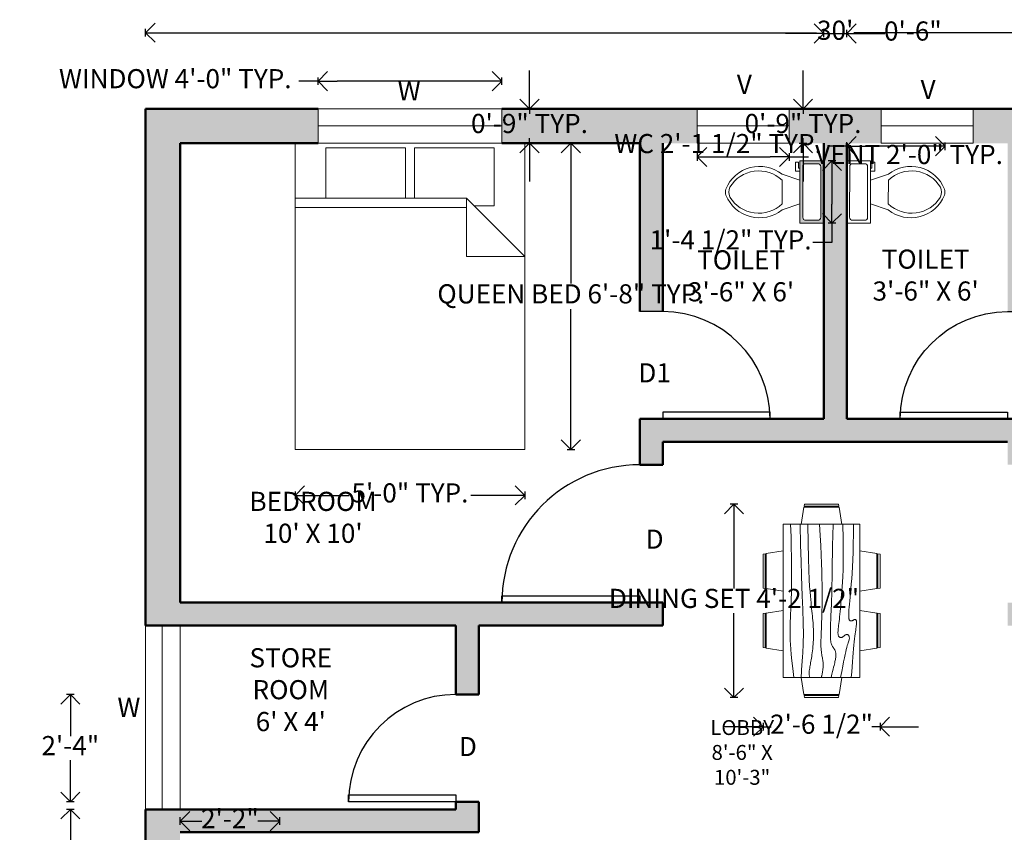
# Model space of a CAD drawing. Units: inches. Extents: x 2691 to 3149, y 584 to 962.
# Tile 2 of 3: x 2709 to 2966, y 750 to 962. Entities that reach past the tile are written whole.
import ezdxf

# ---------------------------------------------------------------- set-up
doc = ezdxf.new("R2010")
doc.units = ezdxf.units.IN
for name, color, linetype, lineweight in [('A-ANNO-DIMS', 2, 'Continuous', 18), ('A-ANNO-TEXT', 159, 'Continuous', 18), ('A-AREA-IDEN', 7, 'Continuous', 25), ('A-DOOR', 4, 'Continuous', 25), ('A-FLOR-FIXT', 9, 'Continuous', 18), ('A-FURN', 8, 'Continuous', 18), ('A-GLAZ', 40, 'Continuous', 18), ('A-WALL', 254, 'Continuous', 50), ('A-WALL-PATT', 252, 'Continuous', 13)]:
    doc.layers.add(name, color=color, linetype=linetype, lineweight=lineweight)
doc.styles.get("Standard").update_dxf_attribs({"font": 'arial.ttf'})
doc.dimstyles.new('ISO-25', dxfattribs={"dimtxt": 5, "dimasz": 5, "dimexe": 1, "dimexo": 1, "dimtad": 0, "dimtih": 1, "dimtoh": 1, "dimdec": 1, "dimlunit": 3, "dimtxsty": 'Standard', "dimblk": 'OPEN90', "dimcen": 2.5, "dimclrd": 1, "dimclre": 1, "dimclrt": 1, "dimadec": 0, "dimazin": 0, "dimtfac": 1, "dimtdec": 1, "dimtmove": 0, "dimatfit": 3, "dimfxl": 1, "dimfxlon": 1, "dimarcsym": 0})

# ---------------------------------------------------------------- blocks, each defined once
blk = doc.blocks.new('*U4')
for p, q in [((-28, 0), (-28, -6)), ((0, 0), (0, -6))]:
    blk.add_line(p, q)
blk.add_lwpolyline([(0, 0), (0, 28), (-1.75, 28), (-1.75, 0)], close=True)
blk.add_arc((0, 0), 28, 90, 180)
blk = doc.blocks.new('*U6')
for p, q in [((0, 0), (0, -6)), ((28, 0), (28, -6))]:
    blk.add_line(p, q)
blk.add_lwpolyline([(0, 0), (0, 28), (1.75, 28), (1.75, 0)], close=True)
blk.add_arc((0, 0), 28, 0, 90)
blk = doc.blocks.new('*U3')
for p, q in [((0, 0), (0, -6)), ((36, 0), (36, -6))]:
    blk.add_line(p, q)
blk.add_lwpolyline([(0, 0), (0, 36), (1.75, 36), (1.75, 0)], close=True)
blk.add_arc((0, 0), 36, 0, 90)
blk = doc.blocks.new('Toilet - top')
for p, q in [((9.5, -6), (9.5, -2)), ((-10, -8.5), (-8, -8.5)), ((-10, -9.5), (-10, -8.5)), ((-7, -9.5), (-10, -9.5)), ((-8, -8.5), (-8, -8)), ((-7, -8), (-7, -9.5)), ((-4, -8), (-6, -14)), ((4, -8), (6, -14)), ((4, -14), (-4, -14))]:
    blk.add_line(p, q)
blk.add_lwpolyline([(10.5, -8), (10.5, 0), (-10.5, 0), (-10.5, -8)], close=True)
for points in [[(-9.5, -2), (-9.5, -6)], [(8.5, -1), (-8.5, -1)], [(-8.5, -7), (8.5, -7)]]:
    blk.add_lwpolyline(points)
for centre, radius, start, end in [((-8.62, -1.88), 0.884, 81.8699, 188.1301), ((8.62, -1.88), 0.884, 351.8699, 98.1301), ((-8.62, -6.12), 0.884, 171.8699, 278.1301), ((8.62, -6.12), 0.884, 261.8699, 8.1301), ((3.52, -21.58), 12.17, 141.4691, 247.9714), ((4.2, -21.82), 11.33, 136.3677, 238.9468), ((-3.52, -21.58), 12.17, 292.0284, 38.5307), ((-4.2, -21.82), 11.33, 301.053, 43.6321), ((0, -27.88), 4, 245.7318, 294.2682), ((0, -29), 4, 254.8605, 285.1395)]:
    blk.add_arc(centre, radius, start, end)
blk = doc.blocks.new('Bed - Queen')
for p, q in [((0, -80.00003), (0, 0)), ((0, 0), (59.99999, 0)), ((59.99999, 0), (59.99999, -80.00003)), ((7.99999, -1.2), (28.79998, -1.2)), ((7.99999, -14.4), (7.99999, -1.2)), ((28.79998, -1.2), (28.79998, -14.4)), ((31.19999, -1.2), (51.99999, -1.2)), ((31.19999, -14.4), (31.19999, -1.2)), ((51.99999, -1.2), (51.99999, -16.4)), ((0, -14.4), (44.8, -14.4)), ((59.99999, -29.6), (44.8, -14.4)), ((44.8, -14.4), (44.8, -29.6)), ((44.8, -16.8), (0, -16.8)), ((51.99999, -16.4), (46.79936, -16.4)), ((44.8, -29.6), (59.99999, -29.6)), ((59.99999, -80.00003), (0, -80.00003))]:
    blk.add_line(p, q)
blk = doc.blocks.new('Dining Set - 36 x 72 in.')
for p, q in [((-22.2343, 26.00059), (-23.4847, 17.99762)), ((-22.2304, 26), (-5.7608, 26)), ((-22, 27.5), (-22.1562, 26.50042)), ((-5.8416, 26.5), (-22.1534, 26.5)), ((-22, 27.5), (-6, 27.5)), ((-5.8437, 26.49966), (-6, 27.5)), ((-4.5152, 17.99762), (-5.7655, 25.99926)), ((5.7657, 26.00059), (4.5153, 17.99762)), ((5.7696, 26), (22.2392, 26)), ((6, 27.5), (5.8438, 26.50042)), ((22.1584, 26.5), (5.8466, 26.5)), ((6, 27.5), (22, 27.5)), ((22.1563, 26.49966), (22, 27.5)), ((23.4848, 17.99762), (22.2345, 25.99926)), ((36, 18), (-36, 18)), ((-36, 18), (-36, -18)), ((36, -18), (36, 18)), ((-44.0006, 8.23428), (-35.9976, 9.48474)), ((44.0006, 8.23428), (35.9976, 9.48474)), ((-45.5, 8), (-44.5004, 8.15617)), ((-45.5, 8), (-45.5, -8)), ((-44.5, -8.15843), (-44.5, 8.15338)), ((-44, 8.23041), (-44, -8.23915)), ((44, 8.23041), (44, -8.23915)), ((44.5, -8.15843), (44.5, 8.15338)), ((45.5, 8), (44.5005, 8.15617)), ((45.5, 8), (45.5, -8)), ((-44.4997, -8.15631), (-45.5, -8)), ((-35.9976, -9.48476), (-43.9993, -8.2345)), ((35.9976, -9.48476), (43.9993, -8.2345)), ((44.4997, -8.15631), (45.5, -8)), ((-36, -18), (36, -18)), ((-22.2343, -26.0006), (-23.4847, -17.99762)), ((-4.5152, -17.99762), (-5.7655, -25.99928)), ((5.7657, -26.0006), (4.5153, -17.99762)), ((23.4848, -17.99762), (22.2345, -25.99928)), ((-22.2304, -26), (-5.7608, -26)), ((-22, -27.5), (-22.1562, -26.50044)), ((-5.8416, -26.5), (-22.1534, -26.5)), ((-22, -27.5), (-6, -27.5)), ((-5.8437, -26.49967), (-6, -27.5)), ((5.7696, -26), (22.2392, -26)), ((6, -27.5), (5.8438, -26.50044)), ((22.1584, -26.5), (5.8466, -26.5)), ((6, -27.5), (22, -27.5)), ((22.1563, -26.49967), (22, -27.5))]:
    blk.add_line(p, q)
for points in [[(-36, 15), (-31.1772, 14.97754), (-26.8079, 14.91406), (-22.8538, 14.81543), (-19.276, 14.6875), (-16.0362, 14.53613), (-13.0957, 14.36718), (-10.4159, 14.18652), (-7.9583, 14), (-5.6904, 13.81315), (-3.6035, 13.63021), (-1.6954, 13.45508), (0.0365, 13.29166), (1.5945, 13.14388), (2.9811, 13.01562), (4.1988, 12.9108), (5.25, 12.83333), (6.1393, 12.78613), (6.8802, 12.76823), (7.4883, 12.77767), (7.9792, 12.8125), (8.3685, 12.87077), (8.6719, 12.95052), (8.9049, 13.0498), (9.0833, 13.16666), (9.2205, 13.29899), (9.3216, 13.44401), (9.3895, 13.59879), (9.4271, 13.76041), (9.4373, 13.92594), (9.4232, 14.09245), (9.3875, 14.257), (9.3333, 14.41666), (9.2638, 14.56917), (9.1836, 14.71484), (9.0975, 14.85465), (9.0104, 14.98958), (8.9272, 15.1206), (8.8529, 15.2487), (8.7922, 15.37483), (8.75, 15.5), (8.7305, 15.62467), (8.7344, 15.74739), (8.7617, 15.86621), (8.8125, 15.97916), (8.8867, 16.08431), (8.9844, 16.17968), (9.1055, 16.26334), (9.25, 16.33333), (9.4189, 16.38802), (9.6172, 16.42708), (9.8506, 16.45052), (10.125, 16.45833), (10.4463, 16.45052), (10.8203, 16.42708), (11.2529, 16.38802), (11.75, 16.33333), (12.3184, 16.26318), (12.9694, 16.17838), (13.7151, 16.07991), (14.5677, 15.96875), (15.5395, 15.84586), (16.6426, 15.71224), (17.8893, 15.56884), (19.2917, 15.41666), (20.859, 15.25667), (22.5879, 15.08984), (24.4721, 14.91715), (26.5052, 14.73958), (28.6809, 14.5581), (30.9929, 14.3737), (33.4347, 14.18733), (36, 14)], [(-36, 10), (-28.9766, 10.14274), (-23.1725, 10.20442), (-18.4241, 10.19775), (-14.5677, 10.13541), (-11.4399, 10.03011), (-8.877, 9.89453), (-6.7154, 9.74137), (-4.7917, 9.58333), (-2.9698, 9.43082), (-1.2246, 9.28515), (0.4415, 9.14534), (2.026, 9.01041), (3.5266, 8.87939), (4.9408, 8.7513), (6.266, 8.62516), (7.5, 8.5), (8.6411, 8.37549), (9.6914, 8.2539), (10.6538, 8.13818), (11.5312, 8.03125), (12.3267, 7.93603), (13.043, 7.85547), (13.6831, 7.79248), (14.25, 7.75), (14.7471, 7.7303), (15.1797, 7.73307), (15.5537, 7.75732), (15.875, 7.80208), (16.1494, 7.86637), (16.3828, 7.94922), (16.5811, 8.04964), (16.75, 8.16666), (16.8944, 8.29915), (17.0143, 8.44531), (17.1089, 8.60319), (17.1771, 8.77083), (17.218, 8.94629), (17.2305, 9.1276), (17.2137, 9.31282), (17.1667, 9.5), (17.0895, 9.6875), (16.987, 9.875), (16.8649, 10.0625), (16.7292, 10.25), (16.5856, 10.4375), (16.4401, 10.625), (16.2985, 10.8125), (16.1667, 11), (16.05, 11.18733), (15.9518, 11.3737), (15.8752, 11.5581), (15.8229, 11.73958), (15.798, 11.91715), (15.8034, 12.08984), (15.842, 12.25667), (15.9167, 12.41666), (16.0295, 12.56836), (16.1784, 12.70833), (16.3605, 12.83268), (16.5729, 12.9375), (16.8127, 13.01888), (17.0768, 13.07291), (17.3625, 13.0957), (17.6667, 13.08333), (17.9894, 13.03312), (18.3418, 12.94726), (18.7382, 12.82918), (19.1927, 12.68229), (19.7195, 12.51001), (20.3327, 12.31575), (21.0465, 12.10294), (21.875, 11.875), (22.8357, 11.63354), (23.959, 11.37304), (25.2786, 11.08618), (26.8282, 10.76562), (28.6414, 10.40405), (30.752, 9.99414), (33.1936, 9.52856), (36, 9)], [(-36, 5.5), (-30.7157, 5.3348), (-26.069, 5.20963), (-21.9946, 5.11767), (-18.4271, 5.05208), (-15.3009, 5.00602), (-12.5508, 4.97265), (-10.1112, 4.94515), (-7.9167, 4.91666), (-5.909, 4.88167), (-4.0586, 4.83984), (-2.3429, 4.79215), (-0.7396, 4.73958), (0.7739, 4.6831), (2.22, 4.6237), (3.6213, 4.56233), (5, 4.5), (6.373, 4.43782), (7.7344, 4.3776), (9.0723, 4.32129), (10.375, 4.27083), (11.6309, 4.22819), (12.8281, 4.19531), (13.9551, 4.17415), (15, 4.16666), (15.954, 4.17448), (16.819, 4.19791), (17.6001, 4.23698), (18.3021, 4.29166), (18.9299, 4.36198), (19.4883, 4.44791), (19.9823, 4.54948), (20.4167, 4.66666), (20.7969, 4.79899), (21.1302, 4.94401), (21.4245, 5.09879), (21.6875, 5.26041), (21.9271, 5.42594), (22.1511, 5.59245), (22.3672, 5.757), (22.5834, 5.91666), (22.8065, 6.06868), (23.0404, 6.21093), (23.2879, 6.34147), (23.5521, 6.45833), (23.8358, 6.55957), (24.142, 6.64323), (24.4735, 6.70735), (24.8334, 6.75), (25.2235, 6.76969), (25.642, 6.76692), (26.0858, 6.74267), (26.5521, 6.69791), (27.0379, 6.63362), (27.5404, 6.55078), (28.0565, 6.45036), (28.5834, 6.33333), (29.1242, 6.19987), (29.7071, 6.04687), (30.3661, 5.87044), (31.1354, 5.66666), (32.0493, 5.43164), (33.142, 5.16146), (34.4475, 4.85221), (36, 4.5)], [(-36, -1), (-30.7915, -0.6591), (-26.0195, -0.38216), (-21.6519, -0.16284), (-17.6563, 0.00521), (-14.0005, 0.12833), (-10.6523, 0.21289), (-7.5796, 0.26522), (-4.75, 0.29166), (-2.134, 0.29793), (0.2878, 0.28711), (2.5317, 0.26163), (4.6146, 0.22396), (6.5529, 0.17651), (8.3633, 0.12174), (10.0623, 0.06209), (11.6667, 0), (13.1899, -0.06201), (14.6341, -0.1211), (15.9982, -0.17432), (17.2813, -0.21875), (18.4823, -0.25147), (19.6003, -0.26953), (20.6343, -0.27002), (21.5834, -0.25), (22.4481, -0.20768), (23.2357, -0.14584), (23.9549, -0.06836), (24.6146, 0.02083), (25.2235, 0.11784), (25.7904, 0.21875), (26.3241, 0.31966), (26.8334, 0.41666), (27.3265, 0.50618), (27.8099, 0.58593), (28.2894, 0.65397), (28.7709, 0.70833), (29.2601, 0.74707), (29.763, 0.76823), (30.2855, 0.76985), (30.8334, 0.75), (31.4088, 0.70784), (31.9994, 0.64713), (32.589, 0.57275), (33.1615, 0.48958), (33.7008, 0.4025), (34.1908, 0.3164), (34.6153, 0.23616), (34.9584, 0.16666), (35.2099, 0.11165), (35.3848, 0.07031), (35.504, 0.04069), (35.5886, 0.02083), (35.6594, 0.00879), (35.7377, 0.0026), (35.8442, 0.00032), (36, 0)], [(-36, -6.5), (-27.1843, -6.31267), (-20.084, -6.1263), (-14.469, -5.9419), (-10.1094, -5.76042), (-6.7752, -5.58285), (-4.2363, -5.41016), (-2.2629, -5.24333), (-0.625, -5.08334), (0.8708, -4.93099), (2.2715, -4.78646), (3.5872, -4.64974), (4.8281, -4.52084), (6.0046, -4.39974), (7.127, -4.28646), (8.2053, -4.18099), (9.25, -4.08334), (10.2705, -3.99382), (11.2734, -3.91407), (12.2647, -3.84603), (13.25, -3.79167), (14.2354, -3.75293), (15.2266, -3.73177), (16.2295, -3.73015), (17.25, -3.75), (18.2912, -3.79248), (19.3451, -3.85547), (20.4009, -3.93604), (21.4479, -4.03125), (22.4754, -4.13819), (23.4727, -4.25391), (24.4289, -4.37549), (25.3334, -4.5), (26.1785, -4.62492), (26.9694, -4.74935), (27.7145, -4.87281), (28.4219, -4.99479), (29.1, -5.11483), (29.7572, -5.23242), (30.4016, -5.34709), (31.0417, -5.45834), (31.6837, -5.56437), (32.3262, -5.65821), (32.9658, -5.73153), (33.599, -5.77604), (34.2224, -5.78345), (34.8327, -5.74545), (35.4264, -5.65373), (36, -5.5)], [(-36, -10), (-26.4022, -9.81299), (-18.4675, -9.62891), (-11.9839, -9.45069), (-6.7396, -9.28125), (-2.5226, -9.12354), (0.8789, -8.98047), (3.6769, -8.85498), (6.0833, -8.75), (8.2767, -8.66765), (10.3021, -8.60677), (12.1712, -8.56543), (13.8958, -8.54167), (15.4876, -8.53353), (16.9583, -8.53907), (18.3197, -8.55632), (19.5834, -8.58334), (20.7616, -8.61841), (21.8685, -8.66081), (22.9188, -8.71004), (23.9271, -8.76563), (24.9081, -8.82707), (25.8763, -8.89388), (26.8465, -8.96558), (27.8334, -9.04167), (28.8474, -9.12118), (29.8828, -9.20117), (30.93, -9.27824), (31.9792, -9.34896), (33.0205, -9.40991), (34.0443, -9.45768), (35.0407, -9.48885), (36, -9.5)], [(-36, -14.5), (-30.0881, -14.33513), (-25.0332, -14.21224), (-20.7312, -14.12647), (-17.0781, -14.07292), (-13.97, -14.04671), (-11.3027, -14.04297), (-8.9724, -14.05681), (-6.875, -14.08334), (-4.9224, -14.11833), (-3.0905, -14.16016), (-1.3709, -14.20785), (0.2448, -14.26042), (1.7647, -14.3169), (3.1973, -14.3763), (4.5507, -14.43767), (5.8333, -14.5), (7.0554, -14.5621), (8.235, -14.62175), (9.3922, -14.67652), (10.5469, -14.72396), (11.7192, -14.76164), (12.929, -14.78711), (14.1965, -14.79794), (15.5417, -14.79167), (16.9933, -14.76424), (18.6152, -14.70508), (20.4804, -14.60197), (22.6615, -14.44271), (25.2312, -14.21509), (28.2624, -13.9069), (31.8277, -13.50594), (36, -13)]]:
    blk.add_lwpolyline(points)
blk = doc.blocks.new('_Open90')
at = {"color": 0, "linetype": 'ByBlock', "lineweight": -2}
for p, q in [((0, 0), (-1, 0)), ((-0.5, 0.5), (0, 0)), ((0, 0), (-0.5, -0.5))]:
    blk.add_line(p, q, dxfattribs=at)
blk = doc.blocks.new('*D15')
at = {"layer": 'A-ANNO-DIMS', "color": 0, "lineweight": -2, "transparency": 16777216}
for p, q in [((2741.63, 957.65), (2741.63, 959.65)), ((3101.65, 957.65), (3101.65, 959.65)), ((2746.63, 958.65), (2916.78, 958.65)), ((3096.65, 958.65), (2926.51, 958.65))]:
    blk.add_line(p, q, dxfattribs=at)
at = {"layer": 'Defpoints', "color": 0, "transparency": 16777216}
for p in [(2741.63, 958.65), (2741.63, 938.8), (3101.65, 938.8)]:
    blk.add_point(p, dxfattribs=at)
at = {"layer": 'A-ANNO-DIMS', "color": 0, "lineweight": -2, "transparency": 16777216, "xscale": 5, "yscale": 5, "zscale": 5, "rotation": 180}
blk.add_blockref('_Open90', (2741.63, 958.65), dxfattribs=at)
at = {"layer": 'A-ANNO-DIMS', "color": 0, "lineweight": -2, "transparency": 16777216, "xscale": 5, "yscale": 5, "zscale": 5}
blk.add_blockref('_Open90', (3101.65, 958.65), dxfattribs=at)
at = {"layer": 'A-ANNO-DIMS', "color": 0, "transparency": 16777216, "insert": (2921.64, 958.65), "char_height": 5, "attachment_point": 5}
blk.add_mtext("30'", dxfattribs=at)
blk = doc.blocks.new('WIN-48IN')
for p, q in [((0, 0), (0, 48)), ((0, 48), (9, 48)), ((4.5, 48), (4.5, 0)), ((9, 0), (9, 48)), ((0, 0), (9, 0))]:
    blk.add_line(p, q)
blk = doc.blocks.new('VENT-24IN')
for p, q in [((0, 0), (0, 9)), ((24, 0), (24, 9)), ((0, 4.5), (24, 4.5)), ((24, 0), (0, 0))]:
    blk.add_line(p, q)
blk = doc.blocks.new('*D20')
at = {"layer": 'A-ANNO-DIMS', "color": 1, "lineweight": -2, "transparency": 16777216}
for p, q in [((2786.63, 946), (2781.63, 946)), ((2786.63, 945), (2786.63, 947)), ((2829.63, 946), (2791.63, 946)), ((2834.63, 945), (2834.63, 947))]:
    blk.add_line(p, q, dxfattribs=at)
at = {"layer": 'Defpoints', "color": 0, "transparency": 16777216}
for p in [(2786.63, 946), (2786.63, 938.8), (2834.63, 938.8)]:
    blk.add_point(p, dxfattribs=at)
at = {"layer": 'A-ANNO-DIMS', "color": 1, "lineweight": -2, "transparency": 16777216, "xscale": 5, "yscale": 5, "zscale": 5}
for p, rotation in [((2786.63, 946), 180.0000000000023), ((2834.63, 946), 2.3181e-12)]:
    blk.add_blockref('_Open90', p, dxfattribs=dict(at, rotation=rotation))
at = {"layer": 'A-ANNO-DIMS', "color": 1, "transparency": 16777216, "insert": (2749.37, 946), "char_height": 5, "attachment_point": 5}
blk.add_mtext('WINDOW 4\'-0" TYP.', dxfattribs=at)
blk = doc.blocks.new('*D21')
at = {"layer": 'A-ANNO-DIMS', "color": 1, "lineweight": -2, "transparency": 16777216}
for p, q in [((2841.83, 943.8), (2841.83, 948.8)), ((2840.83, 938.8), (2842.83, 938.8)), ((2841.83, 938.8), (2841.83, 937.48)), ((2841.83, 929.8), (2841.83, 931.12)), ((2840.83, 929.8), (2842.83, 929.8)), ((2841.83, 924.8), (2841.83, 919.8))]:
    blk.add_line(p, q, dxfattribs=at)
at = {"layer": 'Defpoints', "color": 0, "transparency": 16777216}
for p in [(2834.63, 938.8), (2841.83, 938.8), (2834.63, 929.8)]:
    blk.add_point(p, dxfattribs=at)
at = {"layer": 'A-ANNO-DIMS', "color": 1, "lineweight": -2, "transparency": 16777216, "xscale": 5, "yscale": 5, "zscale": 5}
for p, rotation in [((2841.83, 938.8), 270), ((2841.83, 929.8), 90)]:
    blk.add_blockref('_Open90', p, dxfattribs=dict(at, rotation=rotation))
at = {"layer": 'A-ANNO-DIMS', "color": 1, "transparency": 16777216, "insert": (2841.83, 934.3), "char_height": 5, "attachment_point": 5}
blk.add_mtext('0\'-9" TYP.', dxfattribs=at)
blk = doc.blocks.new('*D24')
at = {"layer": 'A-ANNO-DIMS', "color": 1, "lineweight": -2, "transparency": 16777216}
for p, q in [((2851.63, 929.8), (2853.63, 929.8)), ((2852.63, 924.8), (2852.63, 893.16)), ((2852.63, 854.8), (2852.63, 886.43)), ((2851.63, 849.8), (2853.63, 849.8))]:
    blk.add_line(p, q, dxfattribs=at)
at = {"layer": 'Defpoints', "color": 0, "transparency": 16777216}
for p in [(2840.63, 929.8), (2852.63, 929.8), (2840.63, 849.8)]:
    blk.add_point(p, dxfattribs=at)
at = {"layer": 'A-ANNO-DIMS', "color": 1, "lineweight": -2, "transparency": 16777216, "xscale": 5, "yscale": 5, "zscale": 5}
for p, rotation in [((2852.63, 929.8), 90), ((2852.63, 849.8), 270)]:
    blk.add_blockref('_Open90', p, dxfattribs=dict(at, rotation=rotation))
at = {"layer": 'A-ANNO-DIMS', "color": 1, "transparency": 16777216, "insert": (2852.63, 889.8), "char_height": 5, "attachment_point": 5}
blk.add_mtext('QUEEN BED 6\'-8" TYP.', dxfattribs=at)
blk = doc.blocks.new('*D25')
at = {"layer": 'A-ANNO-DIMS', "color": 1, "lineweight": -2, "transparency": 16777216}
for p, q in [((2780.63, 838.8), (2780.63, 836.8)), ((2840.63, 838.8), (2840.63, 836.8)), ((2785.63, 837.8), (2794.77, 837.8)), ((2835.63, 837.8), (2826.5, 837.8))]:
    blk.add_line(p, q, dxfattribs=at)
at = {"layer": 'Defpoints', "color": 0, "transparency": 16777216}
for p in [(2780.63, 849.8), (2840.63, 849.8), (2840.63, 837.8)]:
    blk.add_point(p, dxfattribs=at)
at = {"layer": 'A-ANNO-DIMS', "color": 1, "lineweight": -2, "transparency": 16777216, "xscale": 5, "yscale": 5, "zscale": 5, "rotation": 180}
blk.add_blockref('_Open90', (2780.63, 837.8), dxfattribs=at)
at = {"layer": 'A-ANNO-DIMS', "color": 1, "lineweight": -2, "transparency": 16777216, "xscale": 5, "yscale": 5, "zscale": 5}
blk.add_blockref('_Open90', (2840.63, 837.8), dxfattribs=at)
at = {"layer": 'A-ANNO-DIMS', "color": 1, "transparency": 16777216, "insert": (2810.63, 837.8), "char_height": 5, "attachment_point": 5}
blk.add_mtext('5\'-0" TYP.', dxfattribs=at)
blk = doc.blocks.new('*D28')
at = {"layer": 'A-ANNO-DIMS', "color": 1, "lineweight": -2, "transparency": 16777216}
for p, q in [((2924.64, 929.04), (2919.64, 929.05)), ((2924.64, 928.04), (2924.64, 930.04)), ((2945.3, 929.03), (2929.64, 929.04)), ((2950.3, 928.02), (2950.3, 930.02))]:
    blk.add_line(p, q, dxfattribs=at)
at = {"layer": 'Defpoints', "color": 0, "transparency": 16777216}
for p in [(2924.64, 929.04), (2924.64, 925.2), (2950.3, 925.18)]:
    blk.add_point(p, dxfattribs=at)
at = {"layer": 'A-ANNO-DIMS', "color": 1, "lineweight": -2, "transparency": 16777216, "xscale": 5, "yscale": 5, "zscale": 5}
for p, rotation in [((2924.64, 929.04), 179.9552121348343), ((2950.3, 929.02), 359.9552121348344)]:
    blk.add_blockref('_Open90', p, dxfattribs=dict(at, rotation=rotation))
at = {"layer": 'A-ANNO-DIMS', "color": 1, "transparency": 16777216, "insert": (2891.06, 929.05), "char_height": 5, "attachment_point": 5}
blk.add_mtext('WC 2\'-1 1/2" TYP.', dxfattribs=at)
blk = doc.blocks.new('*D29')
at = {"layer": 'A-ANNO-DIMS', "color": 1, "lineweight": -2, "transparency": 16777216}
for p, q in [((2921.79, 925.2), (2919.79, 925.2)), ((2920.79, 920.2), (2920.78, 913.89)), ((2921.78, 908.89), (2919.78, 908.89)), ((2920.78, 908.89), (2920.77, 903.89)), ((2920.77, 903.89), (2915.77, 903.89))]:
    blk.add_line(p, q, dxfattribs=at)
at = {"layer": 'Defpoints', "color": 0, "transparency": 16777216}
for p in [(2924.64, 925.2), (2920.78, 908.89), (2924.63, 908.89)]:
    blk.add_point(p, dxfattribs=at)
at = {"layer": 'A-ANNO-DIMS', "color": 1, "lineweight": -2, "transparency": 16777216, "xscale": 5, "yscale": 5, "zscale": 5}
for p, rotation in [((2920.79, 925.2), 89.955212134835), ((2920.78, 908.89), 269.955212134835)]:
    blk.add_blockref('_Open90', p, dxfattribs=dict(at, rotation=rotation))
at = {"layer": 'A-ANNO-DIMS', "color": 1, "transparency": 16777216, "insert": (2894.32, 903.89), "char_height": 5, "attachment_point": 5}
blk.add_mtext('1\'-4 1/2" TYP.', dxfattribs=at)
blk = doc.blocks.new('*D30')
at = {"layer": 'A-ANNO-DIMS', "color": 1, "lineweight": -2, "transparency": 16777216}
for p, q in [((2885.63, 927.2), (2885.63, 925.2)), ((2890.63, 926.2), (2904.63, 926.2)), ((2909.63, 927.2), (2909.63, 925.2)), ((2909.63, 926.2), (2914.63, 926.2))]:
    blk.add_line(p, q, dxfattribs=at)
at = {"layer": 'Defpoints', "color": 0, "transparency": 16777216}
for p in [(2885.63, 929.8), (2909.63, 929.8), (2909.63, 926.2)]:
    blk.add_point(p, dxfattribs=at)
at = {"layer": 'A-ANNO-DIMS', "color": 1, "lineweight": -2, "transparency": 16777216, "xscale": 5, "yscale": 5, "zscale": 5, "rotation": 180}
blk.add_blockref('_Open90', (2885.63, 926.2), dxfattribs=at)
at = {"layer": 'A-ANNO-DIMS', "color": 1, "lineweight": -2, "transparency": 16777216, "xscale": 5, "yscale": 5, "zscale": 5}
blk.add_blockref('_Open90', (2909.63, 926.2), dxfattribs=at)
at = {"layer": 'A-ANNO-DIMS', "color": 1, "transparency": 16777216, "insert": (2940.91, 926.2), "char_height": 5, "attachment_point": 5}
blk.add_mtext('VENT 2\'-0" TYP.', dxfattribs=at)
blk = doc.blocks.new('*D31')
at = {"layer": 'A-ANNO-DIMS', "color": 1, "lineweight": -2, "transparency": 16777216}
for p, q in [((2913.23, 943.8), (2913.23, 948.8)), ((2912.23, 938.8), (2914.23, 938.8)), ((2913.23, 938.8), (2913.23, 937.48)), ((2913.23, 929.8), (2913.23, 931.12)), ((2912.23, 929.8), (2914.23, 929.8)), ((2913.23, 924.8), (2913.23, 919.8))]:
    blk.add_line(p, q, dxfattribs=at)
at = {"layer": 'Defpoints', "color": 0, "transparency": 16777216}
for p in [(2909.63, 938.8), (2913.23, 938.8), (2909.63, 929.8)]:
    blk.add_point(p, dxfattribs=at)
at = {"layer": 'A-ANNO-DIMS', "color": 1, "lineweight": -2, "transparency": 16777216, "xscale": 5, "yscale": 5, "zscale": 5}
for p, rotation in [((2913.23, 938.8), 270), ((2913.23, 929.8), 90)]:
    blk.add_blockref('_Open90', p, dxfattribs=dict(at, rotation=rotation))
at = {"layer": 'A-ANNO-DIMS', "color": 1, "transparency": 16777216, "insert": (2913.23, 934.3), "char_height": 5, "attachment_point": 5}
blk.add_mtext('0\'-9" TYP.', dxfattribs=at)
blk = doc.blocks.new('*D39')
at = {"layer": 'A-ANNO-DIMS', "color": 1, "lineweight": -2, "transparency": 16777216}
for p, q in [((2750.63, 751.73), (2750.63, 753.73)), ((2776.63, 751.73), (2776.63, 753.73)), ((2755.63, 752.73), (2756.32, 752.73)), ((2771.63, 752.73), (2770.95, 752.73))]:
    blk.add_line(p, q, dxfattribs=at)
at = {"layer": 'Defpoints', "color": 0, "transparency": 16777216}
for p in [(2750.63, 752.73), (2750.63, 748.23), (2776.63, 748.23)]:
    blk.add_point(p, dxfattribs=at)
at = {"layer": 'A-ANNO-DIMS', "color": 1, "lineweight": -2, "transparency": 16777216, "xscale": 5, "yscale": 5, "zscale": 5, "rotation": 180}
blk.add_blockref('_Open90', (2750.63, 752.73), dxfattribs=at)
at = {"layer": 'A-ANNO-DIMS', "color": 1, "lineweight": -2, "transparency": 16777216, "xscale": 5, "yscale": 5, "zscale": 5}
blk.add_blockref('_Open90', (2776.63, 752.73), dxfattribs=at)
at = {"layer": 'A-ANNO-DIMS', "color": 1, "transparency": 16777216, "insert": (2763.63, 752.73), "char_height": 5, "attachment_point": 5}
blk.add_mtext('2\'-2"', dxfattribs=at)
blk = doc.blocks.new('*D40')
at = {"layer": 'A-ANNO-DIMS', "color": 1, "lineweight": -2, "transparency": 16777216}
for p, q in [((2896.21, 835.52), (2894.21, 835.52)), ((2895.21, 830.52), (2895.21, 813.46)), ((2895.21, 789.98), (2895.21, 807.04)), ((2896.21, 784.98), (2894.21, 784.98))]:
    blk.add_line(p, q, dxfattribs=at)
at = {"layer": 'Defpoints', "color": 0, "transparency": 16777216}
for p in [(2902.79, 835.52), (2895.21, 784.98), (2902.79, 784.98)]:
    blk.add_point(p, dxfattribs=at)
at = {"layer": 'A-ANNO-DIMS', "color": 1, "lineweight": -2, "transparency": 16777216, "xscale": 5, "yscale": 5, "zscale": 5}
for p, rotation in [((2895.21, 835.52), 90), ((2895.21, 784.98), 270)]:
    blk.add_blockref('_Open90', p, dxfattribs=dict(at, rotation=rotation))
at = {"layer": 'A-ANNO-DIMS', "color": 1, "transparency": 16777216, "insert": (2895.21, 810.25), "char_height": 5, "attachment_point": 5}
blk.add_mtext('DINING SET 4\'-2 1/2"', dxfattribs=at)
blk = doc.blocks.new('*D41')
at = {"layer": 'A-ANNO-DIMS', "color": 1, "lineweight": -2, "transparency": 16777216}
for p, q in [((2897.79, 777.39), (2892.79, 777.39)), ((2902.79, 778.39), (2902.79, 776.39)), ((2902.79, 777.39), (2904.92, 777.39)), ((2933.34, 777.39), (2931.2, 777.39)), ((2933.34, 778.39), (2933.34, 776.39)), ((2938.34, 777.39), (2943.34, 777.39))]:
    blk.add_line(p, q, dxfattribs=at)
at = {"layer": 'Defpoints', "color": 0, "transparency": 16777216}
for p in [(2902.79, 784.98), (2933.34, 784.98), (2933.34, 777.39)]:
    blk.add_point(p, dxfattribs=at)
at = {"layer": 'A-ANNO-DIMS', "color": 1, "lineweight": -2, "transparency": 16777216, "xscale": 5, "yscale": 5, "zscale": 5}
blk.add_blockref('_Open90', (2902.79, 777.39), dxfattribs=at)
at = {"layer": 'A-ANNO-DIMS', "color": 1, "lineweight": -2, "transparency": 16777216, "xscale": 5, "yscale": 5, "zscale": 5, "rotation": 180}
blk.add_blockref('_Open90', (2933.34, 777.39), dxfattribs=at)
at = {"layer": 'A-ANNO-DIMS', "color": 1, "transparency": 16777216, "insert": (2918.06, 777.39), "char_height": 5, "attachment_point": 5}
blk.add_mtext('2\'-6 1/2"', dxfattribs=at)
blk = doc.blocks.new('*D42')
at = {"layer": 'A-ANNO-DIMS', "color": 1, "lineweight": -2, "transparency": 16777216}
for p, q in [((2750.63, 592.67), (2750.63, 590.67)), ((2755.63, 591.67), (2761.36, 591.67)), ((2781.63, 591.67), (2775.9, 591.67)), ((2786.63, 592.67), (2786.63, 590.67))]:
    blk.add_line(p, q, dxfattribs=at)
at = {"layer": 'Defpoints', "color": 0, "transparency": 16777216}
for p in [(2750.63, 929.8), (2786.63, 929.8), (2786.63, 591.67)]:
    blk.add_point(p, dxfattribs=at)
at = {"layer": 'A-ANNO-DIMS', "color": 1, "lineweight": -2, "transparency": 16777216, "xscale": 5, "yscale": 5, "zscale": 5, "rotation": 180}
blk.add_blockref('_Open90', (2750.63, 591.67), dxfattribs=at)
at = {"layer": 'A-ANNO-DIMS', "color": 1, "lineweight": -2, "transparency": 16777216, "xscale": 5, "yscale": 5, "zscale": 5}
blk.add_blockref('_Open90', (2786.63, 591.67), dxfattribs=at)
at = {"layer": 'A-ANNO-DIMS', "color": 1, "transparency": 16777216, "insert": (2768.63, 591.67), "char_height": 5, "attachment_point": 5}
blk.add_mtext('3\'-0"', dxfattribs=at)
blk = doc.blocks.new('*D43')
at = {"layer": 'A-ANNO-DIMS', "color": 1, "lineweight": -2, "transparency": 16777216}
for p, q in [((2871.63, 591.67), (2866.63, 591.67)), ((2876.63, 592.67), (2876.63, 590.67)), ((2876.63, 591.67), (2885.63, 591.67)), ((2885.63, 592.67), (2885.63, 590.67)), ((2890.63, 591.67), (2895.63, 591.67))]:
    blk.add_line(p, q, dxfattribs=at)
at = {"layer": 'Defpoints', "color": 0, "transparency": 16777216}
for p in [(2876.63, 929.8), (2885.63, 929.8), (2885.63, 591.67)]:
    blk.add_point(p, dxfattribs=at)
at = {"layer": 'A-ANNO-DIMS', "color": 1, "lineweight": -2, "transparency": 16777216, "xscale": 5, "yscale": 5, "zscale": 5}
blk.add_blockref('_Open90', (2876.63, 591.67), dxfattribs=at)
at = {"layer": 'A-ANNO-DIMS', "color": 1, "lineweight": -2, "transparency": 16777216, "xscale": 5, "yscale": 5, "zscale": 5, "rotation": 180}
blk.add_blockref('_Open90', (2885.63, 591.67), dxfattribs=at)
at = {"layer": 'A-ANNO-DIMS', "color": 1, "transparency": 16777216, "insert": (2902.9, 591.67), "char_height": 5, "attachment_point": 5}
blk.add_mtext('0\'-9"', dxfattribs=at)
blk = doc.blocks.new('*D46')
at = {"layer": 'A-ANNO-DIMS', "color": 1, "lineweight": -2, "transparency": 16777216}
for p, q in [((2722.98, 755.8), (2720.98, 755.8)), ((2721.98, 750.8), (2721.98, 738.76)), ((2721.98, 720.3), (2721.98, 732.34)), ((2722.98, 715.3), (2720.98, 715.3))]:
    blk.add_line(p, q, dxfattribs=at)
at = {"layer": 'Defpoints', "color": 0, "transparency": 16777216}
for p in [(2721.98, 755.8), (2741.63, 755.8), (2741.63, 715.3)]:
    blk.add_point(p, dxfattribs=at)
at = {"layer": 'A-ANNO-DIMS', "color": 1, "lineweight": -2, "transparency": 16777216, "xscale": 5, "yscale": 5, "zscale": 5}
for p, rotation in [((2721.98, 755.8), 90), ((2721.98, 715.3), 270)]:
    blk.add_blockref('_Open90', p, dxfattribs=dict(at, rotation=rotation))
at = {"layer": 'A-ANNO-DIMS', "color": 1, "transparency": 16777216, "insert": (2721.98, 735.55), "char_height": 5, "attachment_point": 5}
blk.add_mtext('3\'-4 1/2"', dxfattribs=at)
blk = doc.blocks.new('*D50')
at = {"layer": 'A-ANNO-DIMS', "color": 1, "lineweight": -2, "transparency": 16777216}
for p, q in [((2876.63, 592.67), (2876.63, 590.67)), ((2881.63, 591.67), (2883.32, 591.67)), ((2899.63, 591.67), (2897.95, 591.67)), ((2904.63, 592.67), (2904.63, 590.67))]:
    blk.add_line(p, q, dxfattribs=at)
at = {"layer": 'Defpoints', "color": 0, "transparency": 16777216}
for p in [(2876.63, 857.8), (2904.63, 857.8), (2904.63, 591.67)]:
    blk.add_point(p, dxfattribs=at)
at = {"layer": 'A-ANNO-DIMS', "color": 1, "lineweight": -2, "transparency": 16777216, "xscale": 5, "yscale": 5, "zscale": 5, "rotation": 180}
blk.add_blockref('_Open90', (2876.63, 591.67), dxfattribs=at)
at = {"layer": 'A-ANNO-DIMS', "color": 1, "lineweight": -2, "transparency": 16777216, "xscale": 5, "yscale": 5, "zscale": 5}
blk.add_blockref('_Open90', (2904.63, 591.67), dxfattribs=at)
at = {"layer": 'A-ANNO-DIMS', "color": 1, "transparency": 16777216, "insert": (2890.63, 591.67), "char_height": 5, "attachment_point": 5}
blk.add_mtext('2\'-4"', dxfattribs=at)
blk = doc.blocks.new('*D51')
at = {"layer": 'A-ANNO-DIMS', "color": 1, "lineweight": -2, "transparency": 16777216}
for p, q in [((2722.98, 785.8), (2720.98, 785.8)), ((2721.98, 780.8), (2721.98, 774.93)), ((2721.98, 762.8), (2721.98, 768.66)), ((2722.98, 757.8), (2720.98, 757.8))]:
    blk.add_line(p, q, dxfattribs=at)
at = {"layer": 'Defpoints', "color": 0, "transparency": 16777216}
for p in [(2721.98, 785.8), (2822.63, 785.8), (2822.63, 757.8)]:
    blk.add_point(p, dxfattribs=at)
at = {"layer": 'A-ANNO-DIMS', "color": 1, "lineweight": -2, "transparency": 16777216, "xscale": 5, "yscale": 5, "zscale": 5}
for p, rotation in [((2721.98, 785.8), 90), ((2721.98, 757.8), 270)]:
    blk.add_blockref('_Open90', p, dxfattribs=dict(at, rotation=rotation))
at = {"layer": 'A-ANNO-DIMS', "color": 1, "transparency": 16777216, "insert": (2721.98, 771.8), "char_height": 5, "attachment_point": 5}
blk.add_mtext('2\'-4"', dxfattribs=at)
blk = doc.blocks.new('*D53')
at = {"layer": 'A-ANNO-DIMS', "color": 1, "lineweight": -2, "transparency": 16777216}
for p, q in [((2918.63, 957.45), (2918.63, 959.45)), ((2924.63, 957.45), (2924.63, 959.45)), ((2913.63, 958.45), (2908.63, 958.45)), ((2918.63, 958.45), (2924.63, 958.45)), ((2929.63, 958.45), (2934.63, 958.45))]:
    blk.add_line(p, q, dxfattribs=at)
at = {"layer": 'Defpoints', "color": 0, "transparency": 16777216}
for p in [(2924.63, 958.45), (2918.63, 929.8), (2924.63, 929.8)]:
    blk.add_point(p, dxfattribs=at)
at = {"layer": 'A-ANNO-DIMS', "color": 1, "lineweight": -2, "transparency": 16777216, "xscale": 5, "yscale": 5, "zscale": 5}
blk.add_blockref('_Open90', (2918.63, 958.45), dxfattribs=at)
at = {"layer": 'A-ANNO-DIMS', "color": 1, "lineweight": -2, "transparency": 16777216, "xscale": 5, "yscale": 5, "zscale": 5, "rotation": 180}
blk.add_blockref('_Open90', (2924.63, 958.45), dxfattribs=at)
at = {"layer": 'A-ANNO-DIMS', "color": 1, "transparency": 16777216, "insert": (2941.9, 958.45), "char_height": 5, "attachment_point": 5}
blk.add_mtext('0\'-6"', dxfattribs=at)

msp = doc.modelspace()

# ---------------------------------------------------------------- hatches: boundary and pattern name
at = {"layer": 'A-WALL-PATT'}
h = msp.add_hatch(color=256, dxfattribs=at)
h.dxf.hatch_style = 1
h.paths.add_polyline_path([(2786.63, 938.8), (2741.63, 938.8), (2741.63, 803.8), (2822.63, 803.8), (2822.63, 785.8), (2828.63, 785.8), (2828.63, 803.8), (2876.63, 803.8), (2876.63, 809.8), (2870.63, 809.8), (2834.63, 809.8), (2750.63, 809.8), (2750.63, 929.8), (2786.63, 929.8)])
h.paths.add_polyline_path([(2885.63, 938.8), (2834.63, 938.8), (2834.63, 929.8), (2840.63, 929.8), (2870.63, 929.8), (2870.63, 885.8), (2876.63, 885.8), (2876.63, 929.8), (2885.63, 929.8)])
h.paths.add_polyline_path([(2933.63, 938.8), (2909.63, 938.8), (2909.63, 929.8), (2918.63, 929.8), (2918.63, 908.89), (2918.64, 908.89), (2918.63, 925.2), (2912.41, 925.19), (2912.43, 908.88), (2918.63, 908.89), (2918.63, 925.2), (2918.63, 925.2), (2918.64, 908.89), (2918.63, 857.8), (2870.63, 857.8), (2870.63, 845.8), (2876.63, 845.8), (2876.63, 851.8), (2966.63, 851.8), (2966.63, 845.8), (2972.63, 845.8), (2972.63, 857.8), (2924.63, 857.8), (2924.63, 929.8), (2933.63, 929.8)])
h.paths.add_polyline_path([(2917.85, 923.84), (2917.86, 910.44, -0.414214), (2917.28, 909.66), (2913.98, 909.66, -0.414214), (2913.2, 910.24), (2913.19, 923.64, -0.414214), (2913.77, 924.42), (2917.07, 924.42, -0.414214)], flags=16)
h.paths.add_polyline_path([(3008.63, 938.8), (2957.63, 938.8), (2957.63, 929.8), (2966.63, 929.8), (2966.63, 885.8), (2972.63, 885.8), (2972.63, 929.8), (3008.63, 929.8)])
h.paths.add_polyline_path([(3101.63, 938.8), (3056.63, 938.8), (3056.63, 929.8), (3063.83, 929.8), (3092.63, 929.8), (3092.63, 809.8), (2966.63, 809.8), (2966.63, 803.8), (2972.63, 803.8), (2972.63, 797.8), (2978.63, 797.8), (2978.63, 803.8), (3092.63, 803.8), (3092.63, 749.8), (3101.63, 749.8)])
h.paths.add_polyline_path([(2828.63, 757.8), (2822.63, 757.8), (2822.63, 755.8), (2741.63, 755.8), (2741.63, 715.3), (2750.63, 715.3), (2750.63, 749.8), (2828.63, 749.8)])
h.paths.add_polyline_path([(2870.63, 734.8), (2864.63, 734.8), (2864.63, 647.8), (2750.63, 647.8), (2750.63, 679.3), (2741.63, 679.3), (2741.63, 638.8), (2870.63, 638.8)])
h.paths.add_polyline_path([(2924.63, 680.8), (2924.63, 734.8), (2918.63, 734.8), (2918.63, 638.8), (2924.63, 638.8), (2924.63, 644.8)])
h.paths.add_polyline_path([(3011.63, 647.8), (2978.63, 647.8), (2978.63, 761.8), (2972.63, 761.8), (2972.63, 647.8), (2960.51, 647.8, -0.020861), (2960.63, 644.8), (2960.63, 638.8), (3011.63, 638.8)])
h.paths.add_polyline_path([(3101.63, 701.8), (3092.63, 701.8), (3092.63, 647.8), (3059.63, 647.8), (3059.63, 638.8), (3101.63, 638.8)])

# ---------------------------------------------------------------- linework, layer by layer
at = {"layer": 'A-GLAZ'}
for p, q in [((2741.63, 803.8), (2741.63, 755.8)), ((2745.98, 803.8), (2745.98, 755.8)), ((2750.63, 803.8), (2750.63, 755.8))]:
    msp.add_line(p, q, dxfattribs=at)
at = {"layer": 'A-WALL'}
for p, q in [((2741.63, 938.8), (2741.63, 803.8)), ((2786.63, 938.8), (2741.63, 938.8)), ((3056.63, 938.8), (2834.63, 938.8)), ((2750.63, 929.8), (2750.63, 809.8)), ((2786.63, 929.8), (2750.63, 929.8)), ((2870.63, 929.8), (2834.63, 929.8)), ((2870.63, 929.8), (2870.63, 885.8)), ((2876.63, 929.8), (2876.63, 885.8)), ((2918.63, 929.8), (2918.63, 857.8)), ((2924.63, 857.8), (2924.63, 929.8)), ((2918.63, 857.8), (2870.63, 857.8)), ((2870.63, 857.8), (2870.63, 845.8)), ((2972.63, 857.8), (2924.63, 857.8)), ((2966.63, 851.8), (2876.63, 851.8)), ((2876.63, 851.8), (2876.63, 845.8)), ((2870.63, 845.8), (2876.63, 845.8)), ((2876.63, 809.8), (2750.63, 809.8)), ((2876.63, 803.8), (2876.63, 809.8)), ((2822.63, 803.8), (2741.63, 803.8)), ((2822.63, 803.8), (2822.63, 785.8)), ((2876.63, 803.8), (2828.63, 803.8)), ((2828.63, 803.8), (2828.63, 785.8)), ((2822.63, 785.8), (2828.63, 785.8)), ((2822.63, 755.8), (2741.63, 755.8)), ((2741.63, 755.8), (2741.63, 679.3)), ((2822.63, 757.8), (2828.63, 757.8)), ((2822.63, 757.8), (2822.63, 755.8)), ((2828.63, 757.8), (2828.63, 749.8)), ((2750.63, 749.8), (2828.63, 749.8))]:
    msp.add_line(p, q, dxfattribs=at)

# ---------------------------------------------------------------- block references
at = {"layer": 'A-DOOR'}
for name, p, rotation in [('*U4', (2876.63, 857.8), 270), ('*U3', (2870.63, 809.8), 90), ('*U6', (2822.63, 757.8), 90)]:
    msp.add_blockref(name, p, dxfattribs=dict(at, rotation=rotation))
at = {"layer": 'A-DOOR', "xscale": -1, "rotation": 90}
msp.add_blockref('*U4', (2966.63, 857.8), dxfattribs=at)
at = {"layer": 'A-FLOR-FIXT', "yscale": 0.7765204147620104, "zscale": 0.7765204147620104}
for p, xscale, rotation in [((2918.63, 917.04), 0.7765204147620104, 270.0447878651658), ((2924.63, 917.04), -0.7765204147620104, 89.95521213483418)]:
    msp.add_blockref('Toilet - top', p, dxfattribs=dict(at, xscale=xscale, rotation=rotation))
at = {"layer": 'A-FURN'}
msp.add_blockref('Bed - Queen', (2780.63, 929.8), dxfattribs=at)
at = {"layer": 'A-FURN', "xscale": 0.5554163611919471, "yscale": 0.5554163611919471, "zscale": 0.5554163611919471, "rotation": 270}
msp.add_blockref('Dining Set - 36 x 72 in.', (2918.06, 810.25), dxfattribs=at)
at = {"layer": 'A-GLAZ', "rotation": 90.00000000000225}
msp.add_blockref('WIN-48IN', (2834.63, 929.8), dxfattribs=at)
at = {"layer": 'A-GLAZ'}
for p in [(2885.63, 929.8), (2933.63, 929.8)]:
    msp.add_blockref('VENT-24IN', p, dxfattribs=at)

# ---------------------------------------------------------------- texts
at = {"layer": 'A-ANNO-TEXT', "char_height": 5, "attachment_point": 1}
for s, insert in [('\\pxqc;{W}', (2804.81, 945.95)), ('\\pxqc;{V}', (2892.31, 947.68)), ('\\pxqc;{V}', (2940.27, 946.33)), ('\\pxqc;{D1}', (2868.89, 872.32)), ('\\pxqc;{D}', (2868.89, 828.87)), ('\\pxqc;{W}', (2731.66, 784.96)), ('\\pxqc;{D}', (2820.14, 774.7))]:
    msp.add_mtext_dynamic_manual_height_columns(s, width=11.2162, gutter_width=12.5, heights=[0], dxfattribs=dict(at, insert=insert))
at = {"layer": 'A-AREA-IDEN', "attachment_point": 1}
for s, width, gutter_width, insert, char_height in [('\\pxqc;TOILET\\P3\'-6" X 6\'', 40.8517, 12.5, (2876.63, 901.82), 5), ('\\pxqc;TOILET\\P3\'-6" X 6\'', 33.2562, 12.5, (2928.61, 902.02), 5), ("\\pxqc;BEDROOM\\P10' X 10'", 50.6943, 12.5, (2759.98, 838.74), 5), ("\\pxqc;STORE \\PROOM\\P6' X 4'", 41.1379, 12.5, (2758.96, 797.89), 5), ('\\pxqc;LOBBY\\P8\'-6" X 10\'-3"', 30.7616, 9.74, (2881.96, 779.11), 3.8967)]:
    msp.add_mtext_dynamic_manual_height_columns(s, width=width, gutter_width=gutter_width, heights=[0], dxfattribs=dict(at, insert=insert, char_height=char_height))

# ---------------------------------------------------------------- dimensions: what is measured, and where the dimension line sits
at = {"layer": 'A-ANNO-DIMS'}
for base, p1, p2, override, picture, middle in [((2741.63, 958.65), (3101.65, 938.8), (2741.63, 938.8), {"dimclrd": 0, "dimclre": 0, "dimclrt": 0}, '*D15', (2921.64, 958.65)), ((2924.63, 958.45), (2918.63, 929.8), (2924.63, 929.8), {"dimdec": 1, "dimlfac": 1, "dimrnd": 0, "dimzin": 1, "dimdsep": 46, "dimlunit": 4, "dimfrac": 2}, '*D53', (2941.9, 958.45)), ((2786.63, 591.67), (2750.63, 929.8), (2786.63, 929.8), {"dimdec": 1, "dimlfac": 1, "dimrnd": 0, "dimzin": 1, "dimdsep": 46, "dimlunit": 4, "dimfrac": 2}, '*D42', (2768.63, 591.67)), ((2885.63, 591.67), (2876.63, 929.8), (2885.63, 929.8), {"dimdec": 1, "dimlfac": 1, "dimrnd": 0, "dimzin": 1, "dimdsep": 46, "dimlunit": 4, "dimfrac": 2}, '*D43', (2902.9, 591.67)), ((2904.63, 591.67), (2876.63, 857.8), (2904.63, 857.8), {"dimdec": 1, "dimlfac": 1, "dimrnd": 0, "dimzin": 1, "dimdsep": 46, "dimlunit": 4, "dimfrac": 2}, '*D50', (2890.63, 591.67)), ((2933.3374, 777.3938), (2902.7895, 784.9752), (2933.3374, 784.9752), {"dimdec": 1, "dimlfac": 1, "dimrnd": 0, "dimzin": 1, "dimdsep": 46, "dimlunit": 4, "dimfrac": 2}, '*D41', (2918.0635, 777.3938))]:
    dim = msp.add_linear_dim(base=base, p1=p1, p2=p2, dimstyle='ISO-25', override=override, dxfattribs=at)
    dim.commit()
    dim.dimension.update_dxf_attribs({"geometry": picture, "text_midpoint": middle})
for base, p1, p2, angle, text, picture, middle in [((2786.63, 946), (2834.63, 938.8), (2786.63, 938.8), 180, 'WINDOW <> TYP.', '*D20', (2749.37, 946)), ((2841.83, 938.8), (2834.63, 929.8), (2834.63, 938.8), 90, '<> TYP.', '*D21', (2841.83, 934.3)), ((2913.23, 938.8), (2909.63, 929.8), (2909.63, 938.8), 90, '<> TYP.', '*D31', (2913.23, 934.3)), ((2924.64, 929.04), (2950.3, 925.18), (2924.64, 925.2), 179.9552, 'WC <> TYP.', '*D28', (2891.06, 929.05)), ((2852.63, 929.8), (2840.63, 849.8), (2840.63, 929.8), 90, 'QUEEN BED <> TYP.', '*D24', (2852.63, 889.8)), ((2920.78, 908.89), (2924.64, 925.2), (2924.63, 908.89), 269.9552, '<> TYP.', '*D29', (2894.32, 903.89)), ((2895.21, 784.98), (2902.79, 835.52), (2902.79, 784.98), 270, 'DINING SET <>', '*D40', (2895.21, 810.25))]:
    dim = msp.add_linear_dim(base=base, p1=p1, p2=p2, angle=angle, text=text, dimstyle='ISO-25', override={"dimdec": 1, "dimlfac": 1, "dimrnd": 0, "dimzin": 1, "dimdsep": 46, "dimlunit": 4, "dimfrac": 2}, dxfattribs=at)
    dim.commit()
    dim.dimension.update_dxf_attribs({"geometry": picture, "text_midpoint": middle})
for base, p1, p2, text, picture, middle in [((2909.63, 926.2), (2885.63, 929.8), (2909.63, 929.8), 'VENT <> TYP.', '*D30', (2940.91, 926.2)), ((2840.63, 837.8), (2780.63, 849.8), (2840.63, 849.8), '<> TYP.', '*D25', (2810.63, 837.8))]:
    dim = msp.add_linear_dim(base=base, p1=p1, p2=p2, text=text, dimstyle='ISO-25', override={"dimdec": 1, "dimlfac": 1, "dimrnd": 0, "dimzin": 1, "dimdsep": 46, "dimlunit": 4, "dimfrac": 2}, dxfattribs=at)
    dim.commit()
    dim.dimension.update_dxf_attribs({"geometry": picture, "text_midpoint": middle})
for base, p1, p2, angle, picture, middle in [((2721.98, 785.8), (2822.63, 757.8), (2822.63, 785.8), 90, '*D51', (2721.98, 771.8)), ((2721.98, 755.8), (2741.63, 715.3), (2741.63, 755.8), 90, '*D46', (2721.98, 735.55)), ((2750.63, 752.73), (2776.63, 748.23), (2750.63, 748.23), 180, '*D39', (2763.63, 752.73))]:
    dim = msp.add_linear_dim(base=base, p1=p1, p2=p2, angle=angle, dimstyle='ISO-25', override={"dimdec": 1, "dimlfac": 1, "dimrnd": 0, "dimzin": 1, "dimdsep": 46, "dimlunit": 4, "dimfrac": 2}, dxfattribs=at)
    dim.commit()
    dim.dimension.update_dxf_attribs({"geometry": picture, "text_midpoint": middle})

doc.saveas('drawing.dxf')
